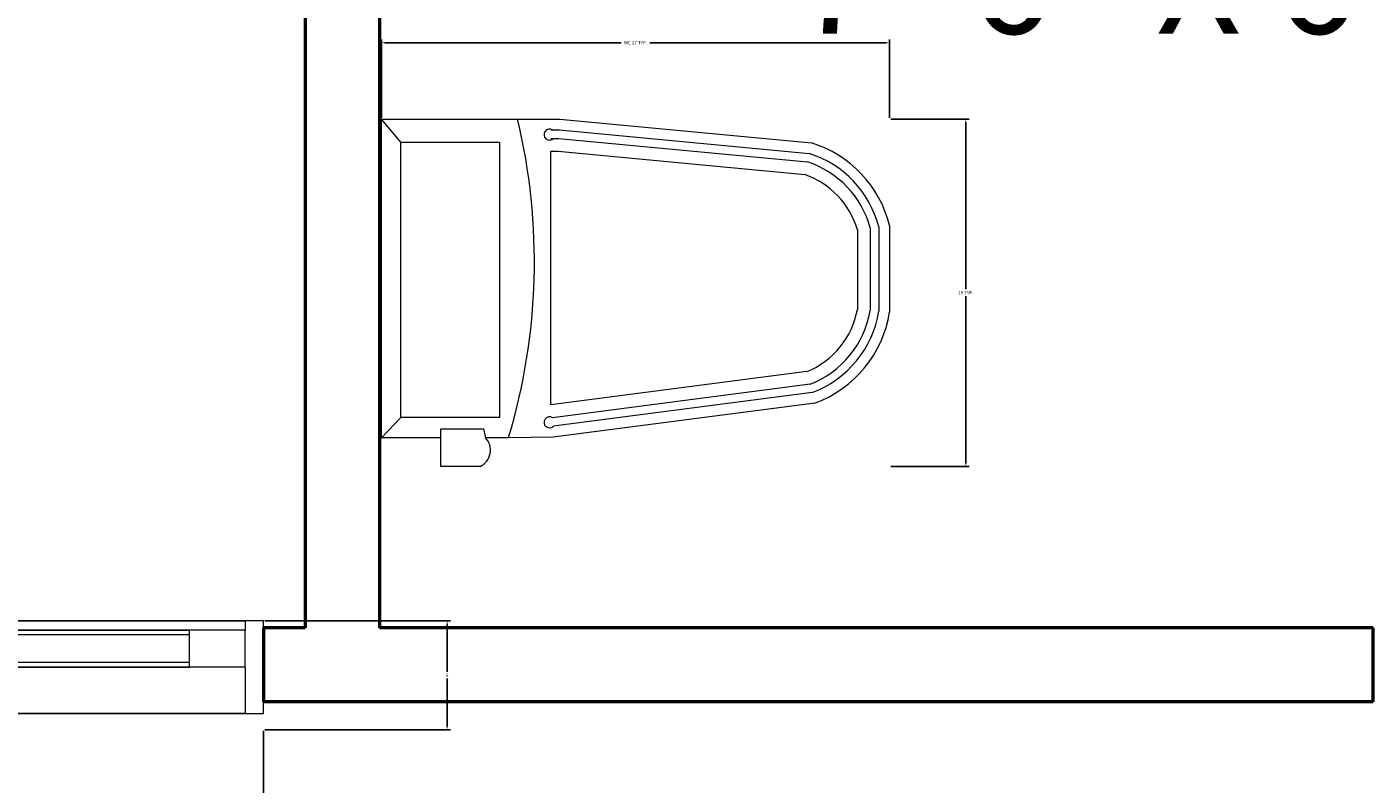
# Model space of a CAD drawing. Units: inches. Extents: x 64 to 1167, y 117 to 939.
# Tile 21 of 56: x 358 to 431, y 777 to 818. Entities that reach past the tile are written whole.
import ezdxf

# ---------------------------------------------------------------- set-up
doc = ezdxf.new("R2010")
doc.units = ezdxf.units.IN
doc.header["$MEASUREMENT"] = 0
for name, color, linetype, lineweight in [('A-ANNO-DIMS', 2, 'Continuous', 18), ('A-ANNO-TEXT', 7, 'Continuous', 25), ('A-DOOR', 4, 'Continuous', 25), ('A-FLOR-FIXT', 8, 'Continuous', 18), ('A-WALL', 7, 'Continuous', 50), ('cut', 6, 'Continuous', 18)]:
    doc.layers.add(name, color=color, linetype=linetype, lineweight=lineweight)
doc.styles.get("Standard").update_dxf_attribs({"font": 'arial.ttf'})
doc.dimstyles.get("Standard").update_dxf_attribs({"dimtxt": 0.18, "dimasz": 0.18, "dimexe": 0.18, "dimexo": 0.0625, "dimgap": 0.09, "dimtad": 0, "dimtih": 1, "dimtoh": 1, "dimdec": 4, "dimzin": 0, "dimdsep": 46, "dimtxsty": 'Standard', "dimcen": 0.09, "dimadec": 0, "dimazin": 0, "dimtfac": 1, "dimtdec": 4, "dimtofl": 0, "dimtmove": 0, "dimatfit": 3, "dimfxl": 1, "dimtolj": 1, "dimtzin": 0, "dimarcsym": 0})

# ---------------------------------------------------------------- blocks, each defined once
blk = doc.blocks.new('A$C2B992F40')
for p, q in [((39.2, 615.2), (39.2, 696.2)), ((39.2, 696.2), (475.7, 696.2)), ((66.8, 669.7), (39.2, 696.2)), ((444.2, 669.7), (475.7, 696.2)), ((475.7, 696.2), (475.7, 509.8)), ((66.8, 534.6), (66.8, 669.7)), ((66.8, 669.7), (444.2, 669.7)), ((444.2, 669.7), (444.2, 534.6)), ((0, 561.3), (0, 615.2)), ((0, 615.2), (51.5, 615.2)), ((51.5, 615.2), (51.5, 556.4)), ((51.5, 556.4), (39.2, 553.9)), ((39.2, 522.1), (39.2, 553.9)), ((40.1, 461.2), (39.2, 522.1)), ((444.2, 534.6), (66.8, 534.6)), ((475.7, 509.8), (475.7, 451.9)), ((86.6, 102.5), (40.1, 461.2)), ((112.5, 109), (66.6, 462.1)), ((84.2, 464.4), (431.5, 464.4)), ((129.7, 113.4), (84.2, 464.4)), ((431.5, 464.4), (431.5, 454)), ((449.2, 464.4), (449.2, 453.2)), ((461, 464.4), (461, 452.6)), ((101, 106.1), (55, 460.6)), ((431.5, 454), (399.6, 116.2)), ((449.2, 453.2), (417, 112.5)), ((461, 452.6), (428.6, 110.1)), ((475.7, 451.9), (443.1, 107.2)), ((324.2, 44.1), (215, 44.1)), ((326.7, 26.5), (213.4, 26.5)), ((330.1, 0), (211.3, 0)), ((328.2, 14.7), (212.5, 14.7))]:
    blk.add_line(p, q)
for centre, radius, start, end in [((22.2, 571.4), 24.4, 204.4997, 314.261), ((280.3, 1327.8), 841, 253.3464, 283.4356), ((60.2, 466.1), 7.56, 328.5293, 226.2699), ((454.4, 466.1), 7.56, 328.5293, 226.2699), ((235.9, 157), 114.8, 202.302, 259.4948), ((291.5, 153.8), 114.4, 286.5809, 340.8155), ((291.5, 153.8), 132.1, 285.4258, 341.7737), ((235.9, 157), 158.9, 200.0551, 261.0752), ((235.9, 157), 144.2, 200.6876, 260.6301), ((235.9, 157), 132.4, 201.2682, 260.2217), ((291.5, 153.8), 143.8, 284.7775, 342.3116), ((291.5, 153.8), 158.5, 284.0717, 342.8974)]:
    blk.add_arc(centre, radius, start, end)
blk = doc.blocks.new('Sliding Glass Door pl')
for p, q in [((28.469, -0.005), (-35.531, -0.005)), ((-0.531, -0.505), (25.469, -0.505)), ((-34.531, -1.13), (-33.878, -1.13)), ((-34.531, -1.13), (-34.531, -1.63)), ((-33.878, -1.13), (-33.878, -1.63)), ((-32.355, -1.13), (-33.878, -1.13)), ((-32.355, -1.13), (-32.355, -1.63)), ((-34.531, -1.63), (-34.281, -1.63)), ((-34.281, -2.38), (-34.281, -1.63)), ((-34.281, -1.63), (-33.878, -1.63)), ((-33.878, -1.63), (-33.781, -1.63)), ((-33.781, -2.38), (-33.781, -1.63)), ((-32.355, -1.63), (-33.781, -1.63)), ((-34.281, -2.38), (-34.531, -2.38)), ((-34.531, -2.505), (-34.531, -2.38)), ((-34.281, -2.38), (-33.781, -2.38)), ((-33.531, -2.38), (-33.781, -2.38)), ((-33.531, -2.505), (-33.531, -2.38)), ((-32.531, -2.505), (-6.531, -2.505)), ((-0.531, -2.505), (25.469, -2.505)), ((-35.531, -5.005), (-34.281, -5.005)), ((-34.531, -4.505), (-34.531, -4.63)), ((-34.531, -4.63), (-34.281, -4.63)), ((-34.281, -4.63), (-33.781, -4.63)), ((-34.281, -4.63), (-34.281, -5.005)), ((-34.281, -5.005), (-34.281, -5.38)), ((-33.781, -4.63), (-33.781, -5.005)), ((-33.781, -4.63), (-33.531, -4.63)), ((-33.781, -5.005), (28.469, -5.005)), ((-33.781, -5.005), (-33.781, -5.38)), ((-33.531, -4.505), (-33.531, -4.63)), ((-32.531, -4.505), (-6.531, -4.505)), ((-34.281, -5.38), (-34.531, -5.38)), ((-34.531, -5.88), (-34.531, -5.38)), ((-34.281, -5.38), (-33.878, -5.38)), ((-33.878, -5.88), (-33.878, -5.38)), ((-33.781, -5.38), (-33.878, -5.38)), ((-33.781, -5.38), (-32.355, -5.38)), ((-32.355, -5.88), (-32.355, -5.38)), ((-34.531, -5.88), (-33.878, -5.88)), ((-33.878, -5.88), (-32.355, -5.88))]:
    blk.add_line(p, q)
at = {"layer": 'cut'}
for p, q in [((-36.531, -0.005), (-36.531, -5.005)), ((-35.531, -0.005), (-36.531, -0.005)), ((-35.531, -2.505), (-35.531, -0.005)), ((-0.531, -0.505), (-3.531, -0.505)), ((-3.531, -2.505), (-3.531, -0.505)), ((-0.531, -0.755), (-0.531, -0.505)), ((28.469, -0.505), (25.469, -0.505)), ((25.469, -0.755), (25.469, -0.505)), ((29.469, -0.005), (28.469, -0.005)), ((28.469, -0.005), (28.469, -0.505)), ((28.469, -2.505), (28.469, -0.505)), ((29.469, -5.005), (29.469, -0.005)), ((25.469, -0.755), (-0.531, -0.755)), ((-0.531, -2.255), (-0.531, -0.755)), ((25.469, -2.255), (25.469, -0.755)), ((-34.531, -2.505), (-35.531, -2.505)), ((-35.531, -4.505), (-35.531, -2.505)), ((-34.531, -2.505), (-33.531, -2.505)), ((-32.531, -2.505), (-33.531, -2.505)), ((-32.531, -2.755), (-32.531, -2.505)), ((-6.531, -2.755), (-32.531, -2.755)), ((-32.531, -4.255), (-32.531, -2.755)), ((-3.531, -2.505), (-6.531, -2.505)), ((-6.531, -2.755), (-6.531, -2.505)), ((-6.531, -4.255), (-6.531, -2.755)), ((-3.531, -4.505), (-3.531, -2.505)), ((-0.531, -2.505), (-3.531, -2.505)), ((25.469, -2.255), (-0.531, -2.255)), ((-0.531, -2.505), (-0.531, -2.255)), ((25.469, -2.505), (25.469, -2.255)), ((28.469, -2.505), (25.469, -2.505)), ((28.469, -2.505), (28.469, -5.005)), ((-6.531, -4.255), (-32.531, -4.255)), ((-32.531, -4.505), (-32.531, -4.255)), ((-6.531, -4.505), (-6.531, -4.255)), ((-36.531, -5.005), (-35.531, -5.005)), ((-35.531, -5.005), (-35.531, -4.505)), ((-34.531, -4.505), (-35.531, -4.505)), ((-33.531, -4.505), (-34.531, -4.505)), ((-32.531, -4.505), (-33.531, -4.505)), ((-3.531, -4.505), (-6.531, -4.505)), ((28.469, -5.005), (29.469, -5.005))]:
    blk.add_line(p, q, dxfattribs=at)
blk = doc.blocks.new('*D66')
at = {"layer": 'A-ANNO-DIMS', "color": 0, "lineweight": -2, "transparency": 16777216}
for p, q in [((377.224, 812.693), (377.224, 816.921)), ((377.404, 816.741), (390.152, 816.741)), ((404.452, 816.741), (391.704, 816.741)), ((404.632, 812.693), (404.632, 816.921))]:
    blk.add_line(p, q, dxfattribs=at)
for points in [[(377.404, 816.771), (377.404, 816.711), (377.224, 816.741)], [(404.452, 816.771), (404.452, 816.711), (404.632, 816.741)]]:
    blk.add_solid(points, dxfattribs=at)
at = {"layer": 'Defpoints', "color": 0, "lineweight": -2, "transparency": 16777216}
for p in [(377.224, 816.741), (377.224, 812.63), (404.632, 812.63)]:
    blk.add_point(p, dxfattribs=at)
at = {"layer": 'A-ANNO-DIMS', "color": 0, "transparency": 16777216, "insert": (390.928, 816.741), "char_height": 0.18, "attachment_point": 5}
blk.add_mtext('\\A1;WC 27 TYP.', dxfattribs=at)
blk = doc.blocks.new('*D67')
at = {"layer": 'A-ANNO-DIMS', "color": 0, "lineweight": -2, "transparency": 16777216}
for p, q in [((404.694, 812.63), (408.923, 812.63)), ((408.743, 812.45), (408.743, 803.448)), ((408.743, 794.083), (408.743, 803.085)), ((404.694, 793.903), (408.923, 793.903))]:
    blk.add_line(p, q, dxfattribs=at)
for points in [[(408.713, 812.45), (408.773, 812.45), (408.743, 812.63)], [(408.713, 794.083), (408.773, 794.083), (408.743, 793.903)]]:
    blk.add_solid(points, dxfattribs=at)
at = {"layer": 'Defpoints', "color": 0, "lineweight": -2, "transparency": 16777216}
for p in [(404.632, 812.63), (408.743, 812.63), (404.632, 793.903)]:
    blk.add_point(p, dxfattribs=at)
at = {"layer": 'A-ANNO-DIMS', "color": 0, "transparency": 16777216, "insert": (408.743, 803.266), "char_height": 0.18, "attachment_point": 5}
blk.add_mtext('\\A1;19 TYP.', dxfattribs=at)
blk = doc.blocks.new('*D94')
at = {"layer": 'A-ANNO-DIMS', "color": 0, "lineweight": -2, "transparency": 16777216}
for p, q in [((304.86, 779.638), (304.86, 769.621)), ((370.86, 779.638), (370.86, 769.621)), ((305.04, 769.801), (336.237, 769.801)), ((370.68, 769.801), (339.483, 769.801))]:
    blk.add_line(p, q, dxfattribs=at)
for points in [[(305.04, 769.831), (305.04, 769.771), (304.86, 769.801)], [(370.68, 769.831), (370.68, 769.771), (370.86, 769.801)]]:
    blk.add_solid(points, dxfattribs=at)
at = {"layer": 'Defpoints', "color": 0, "lineweight": -2, "transparency": 16777216}
for p in [(304.86, 779.701), (370.86, 779.701), (370.86, 769.801)]:
    blk.add_point(p, dxfattribs=at)
at = {"layer": 'A-ANNO-DIMS', "color": 0, "transparency": 16777216, "insert": (337.86, 769.801), "char_height": 0.18, "attachment_point": 5}
blk.add_mtext('\\A1;SLIDING GLASS DOOR 66', dxfattribs=at)
blk = doc.blocks.new('*D95')
at = {"layer": 'A-ANNO-DIMS', "color": 0, "lineweight": -2, "transparency": 16777216}
for p, q in [((370.922, 785.576), (380.94, 785.576)), ((380.76, 785.396), (380.76, 782.82)), ((380.76, 779.881), (380.76, 782.456)), ((370.922, 779.701), (380.94, 779.701))]:
    blk.add_line(p, q, dxfattribs=at)
for points in [[(380.73, 785.396), (380.79, 785.396), (380.76, 785.576)], [(380.73, 779.881), (380.79, 779.881), (380.76, 779.701)]]:
    blk.add_solid(points, dxfattribs=at)
at = {"layer": 'Defpoints', "color": 0, "lineweight": -2, "transparency": 16777216}
for p in [(370.86, 785.576), (380.76, 785.576), (370.86, 779.701)]:
    blk.add_point(p, dxfattribs=at)
at = {"layer": 'A-ANNO-DIMS', "color": 0, "transparency": 16777216, "insert": (380.76, 782.638), "char_height": 0.18, "attachment_point": 5}
blk.add_mtext('\\A1;6', dxfattribs=at)

msp = doc.modelspace()

# ---------------------------------------------------------------- linework, layer by layer
at = {"layer": 'A-WALL'}
for p, q in [((373.107, 847.311), (373.107, 785.2)), ((377.107, 847.311), (377.107, 785.2)), ((373.107, 785.2), (370.86, 785.2)), ((370.86, 785.2), (370.86, 781.2)), ((430.716, 785.2), (377.107, 785.2)), ((430.716, 781.2), (430.716, 785.2)), ((430.716, 781.2), (370.86, 781.2))]:
    msp.add_line(p, q, dxfattribs=at)

# ---------------------------------------------------------------- block references
at = {"layer": 'A-DOOR'}
msp.add_blockref('Sliding Glass Door pl', (341.391, 785.581), dxfattribs=at)
at = {"layer": 'A-FLOR-FIXT', "xscale": 0.0393700787401575, "yscale": 0.0393700787401575, "zscale": 0.0393700787401575, "rotation": 90.00000000001545}
msp.add_blockref('A$C2B992F40', (404.632, 793.903), dxfattribs=at)

# ---------------------------------------------------------------- texts
at = {"layer": 'A-ANNO-TEXT'}
msp.add_text(' 7\'-6" X 6\'-0"', height=5.89263, dxfattribs=at).set_placement((397.637, 817.235))

# ---------------------------------------------------------------- dimensions: what is measured, and where the dimension line sits
at = {"layer": 'A-ANNO-DIMS'}
for base, p1, p2, angle, text, picture, middle in [((377.224, 816.741), (404.632, 812.63), (377.224, 812.63), 180, 'WC <> TYP.', '*D66', (390.928, 816.741)), ((408.743, 812.63), (404.632, 793.903), (404.632, 812.63), 90, '<> TYP.', '*D67', (408.743, 803.266))]:
    dim = msp.add_linear_dim(base=base, p1=p1, p2=p2, angle=angle, text=text, dimstyle='Standard', override={"dimdec": 0, "dimlfac": 1, "dimrnd": 0, "dimzin": 0, "dimdsep": 46, "dimlunit": 2}, dxfattribs=at)
    dim.commit()
    dim.dimension.update_dxf_attribs({"geometry": picture, "text_midpoint": middle})
dim = msp.add_linear_dim(base=(380.76, 785.576), p1=(370.86, 779.701), p2=(370.86, 785.576), angle=90, dimstyle='Standard', override={"dimdec": 0, "dimlfac": 1, "dimrnd": 0, "dimzin": 0, "dimdsep": 46, "dimlunit": 2}, dxfattribs=at)
dim.commit()
dim.dimension.update_dxf_attribs({"geometry": '*D95', "text_midpoint": (380.76, 782.638)})
dim = msp.add_linear_dim(base=(370.86, 769.801), p1=(304.86, 779.701), p2=(370.86, 779.701), text='SLIDING GLASS DOOR <>', dimstyle='Standard', override={"dimdec": 0, "dimlfac": 1, "dimrnd": 0, "dimzin": 0, "dimdsep": 46, "dimlunit": 2}, dxfattribs=at)
dim.commit()
dim.dimension.update_dxf_attribs({"geometry": '*D94', "text_midpoint": (337.86, 769.801)})

doc.saveas('drawing.dxf')
